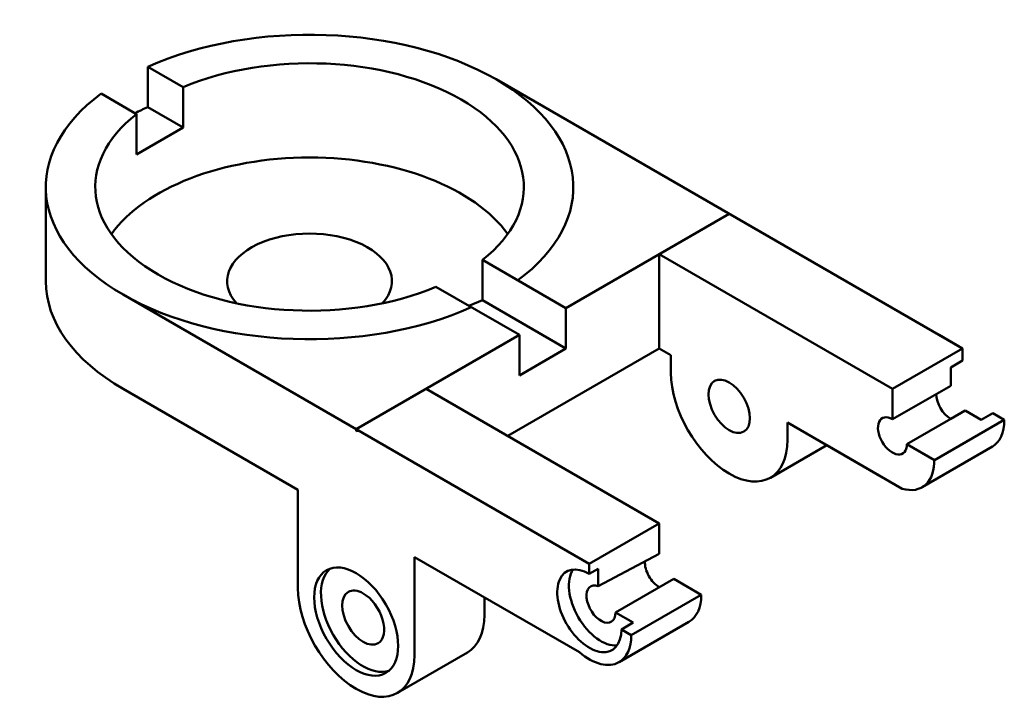
# Model space of a CAD drawing. Units: millimetres. Extents: x 3091 to 3457, y 1409 to 1661.
import ezdxf

# ---------------------------------------------------------------- set-up
doc = ezdxf.new("R2010")
doc.units = ezdxf.units.MM
doc.layers.add('M-OUTL', color=7, linetype='Continuous', lineweight=50)

msp = doc.modelspace()

# ---------------------------------------------------------------- linework, layer by layer
at = {"layer": 'M-OUTL'}
for p, q in [((3151.52, 1635.64), (3138.4, 1643.21)), ((3138.4, 1643.21), (3138.4, 1628.21)), ((3151.52, 1635.64), (3151.52, 1620.64)), ((3267.76, 1638.53), (3440.97, 1538.53)), ((3134.2, 1625.64), (3121.08, 1633.21)), ((3138.4, 1628.21), (3151.52, 1620.64)), ((3134.2, 1625.64), (3134.2, 1610.64)), ((3134.2, 1610.64), (3151.52, 1620.64)), ((3100.5, 1598.53), (3100.5, 1563.53)), ((3354.37, 1588.53), (3293.74, 1553.53)), ((3354.37, 1588.53), (3328.39, 1573.53)), ((3440.97, 1538.53), (3354.37, 1588.53)), ((3328.39, 1573.53), (3414.99, 1523.53)), ((3328.39, 1573.53), (3328.39, 1538.53)), ((3262.76, 1571.41), (3293.74, 1553.53)), ((3262.76, 1571.41), (3262.76, 1556.41)), ((3129.2, 1558.53), (3302.4, 1458.53)), ((3245.44, 1561.41), (3276.42, 1543.53)), ((3262.76, 1556.41), (3257.63, 1554.38)), ((3293.74, 1538.53), (3262.76, 1556.41)), ((3293.74, 1553.53), (3293.74, 1538.53)), ((3276.42, 1543.53), (3215.8, 1508.53)), ((3276.42, 1543.53), (3276.42, 1528.53)), ((3440.97, 1538.53), (3432.31, 1543.53)), ((3328.39, 1538.53), (3272.09, 1506.03)), ((3276.42, 1528.53), (3293.74, 1538.53)), ((3332.72, 1536.03), (3328.39, 1538.53)), ((3440.97, 1538.53), (3414.99, 1523.53)), ((3440.97, 1538.53), (3440.97, 1534.06)), ((3440.97, 1538.53), (3440.97, 1534.06)), ((3332.72, 1529.53), (3332.72, 1536.03)), ((3440.97, 1534.06), (3436.73, 1531.5)), ((3436.73, 1531.5), (3436.69, 1524.7)), ((3129.2, 1523.53), (3194.15, 1486.03)), ((3215.8, 1508.53), (3241.78, 1523.53)), ((3241.78, 1523.53), (3328.39, 1473.53)), ((3436.69, 1524.7), (3414.99, 1512.23)), ((3414.99, 1523.53), (3414.99, 1512.23)), ((3436.64, 1512.32), (3442.01, 1515.42)), ((3447.92, 1512.01), (3442.01, 1515.42)), ((3452.25, 1514.51), (3447.92, 1512.01)), ((3452.25, 1514.51), (3456.56, 1512.03)), ((3376.02, 1504.53), (3376.02, 1511.03)), ((3411.34, 1490.63), (3376.02, 1511.03)), ((3420.36, 1502.92), (3436.64, 1512.32)), ((3430.58, 1497.03), (3456.56, 1512.03)), ((3436.69, 1512.35), (3436.69, 1512.29)), ((3302.4, 1458.53), (3215.8, 1508.53)), ((3215.8, 1508.53), (3215.8, 1507.85)), ((3369.68, 1490.51), (3390.61, 1502.6)), ((3390.61, 1502.6), (3418.64, 1486.42)), ((3430.58, 1497.03), (3420.36, 1502.92)), ((3426.01, 1486.93), (3452.19, 1502.05)), ((3452.19, 1502.05), (3452.19, 1502.05)), ((3430.14, 1497.28), (3430.58, 1497.03)), ((3194.15, 1449.53), (3194.15, 1486.03)), ((3302.4, 1458.53), (3328.39, 1473.53)), ((3328.39, 1473.53), (3328.39, 1462.23)), ((3237.45, 1424.53), (3237.45, 1461.03)), ((3237.45, 1461.03), (3298.76, 1425.63)), ((3305.73, 1450.2), (3328.39, 1462.23)), ((3302.4, 1458.53), (3302.4, 1454.78)), ((3302.4, 1454.78), (3305.73, 1456.7)), ((3305.73, 1456.7), (3305.73, 1450.2)), ((3333.76, 1452.92), (3312.11, 1440.42)), ((3333.76, 1452.92), (3343.97, 1447.03)), ((3263.43, 1439.53), (3263.43, 1446.03)), ((3317.99, 1432.03), (3343.97, 1447.03)), ((3312.11, 1440.42), (3318.64, 1436.65)), ((3313.43, 1421.94), (3339.41, 1436.93)), ((3314.31, 1434.15), (3318.64, 1436.65)), ((3314.31, 1434.15), (3317.99, 1432.03)), ((3316.54, 1436.5), (3316.54, 1436.5)), ((3322.32, 1434.53), (3322.46, 1434.45)), ((3231.11, 1410.51), (3257.09, 1425.51))]:
    msp.add_line(p, q, dxfattribs=at)
for centre, major_axis, start_param, end_param in [((3198.48, 1598.53), (-97.98, 0), 8.764708, 11.655645), ((3198.48, 1598.53), (-79.61, 0), 8.793839, 11.626513), ((3198.48, 1598.53), (-97.98, 0), 5.623115, 8.514052), ((3198.48, 1583.53), (-97.98, 0), 5.372459, 5.435246), ((3198.48, 1598.53), (-79.61, 0), 5.652247, 8.48492), ((3198.48, 1563.53), (-79.61, 0), 9.815385, 12.175764), ((3198.48, 1563.53), (-30.62, 0), 2.658331, 6.766447), ((3198.48, 1563.53), (-97.98, 0), 6.283185, 7.068583), ((3354.37, 1517.03), (15.31, -26.52), 3.926991, 7.068583), ((3436.64, 1518.53), (3.8, -6.58), 3.926991, 5.497787), ((3414.99, 1506.03), (3.8, -6.58), 2.356194, 7.068583), ((3436.64, 1518.53), (3.8, -6.58), 5.497787, 5.507803), ((3440.97, 1521.03), (11.02, -19.09), 6.283185, 7.068583), ((3198.48, 1563.53), (-97.98, 0), 8.031692, 8.041973), ((3414.99, 1506.03), (11.02, -19.09), 5.734038, 7.095989), ((3328.39, 1456.03), (3.8, -6.58), 3.885848, 5.497787), ((3218.3, 1438.47), (11.02, -19.09), 3.255188, 6.169589), ((3302.4, 1441.03), (8.42, -14.59), 2.356194, 7.068583), ((3306.73, 1443.53), (8.42, -14.59), 3.4016, 6.023178), ((3302.4, 1441.03), (11.02, -19.09), 2.328724, 2.328789), ((3306.73, 1443.53), (8.42, -14.59), 8.97317, 8.973311), ((3215.8, 1437.03), (15.31, -26.52), 3.926991, 7.068583), ((3218.4, 1438.53), (5.51, -9.55), 2.356194, 3.141593), ((3306.73, 1443.53), (3.8, -6.58), 2.54516, 7.068583), ((3218.4, 1438.53), (5.51, -9.55), 3.141593, 6.283185), ((3218.4, 1438.53), (5.51, -9.55), 0, 2.356194), ((3328.39, 1456.03), (11.02, -19.09), 6.282629, 7.068583), ((3241.78, 1452.03), (15.31, -26.52), 6.283185, 7.068583), ((3302.4, 1441.03), (-11.02, 19.09), 3.141593, 3.926991), ((3302.4, 1441.03), (-11.02, 19.09), 2.119943, 3.141593)]:
    msp.add_ellipse(centre, major_axis=major_axis, ratio=0.57735, start_param=start_param, end_param=end_param, dxfattribs=at)
for centre, major_axis in [((3354.37, 1517.03), (5.43, -9.41)), ((3215.8, 1437.03), (11.02, -19.09))]:
    msp.add_ellipse(centre, major_axis=major_axis, ratio=0.57735, dxfattribs=at)

doc.saveas('drawing.dxf')
